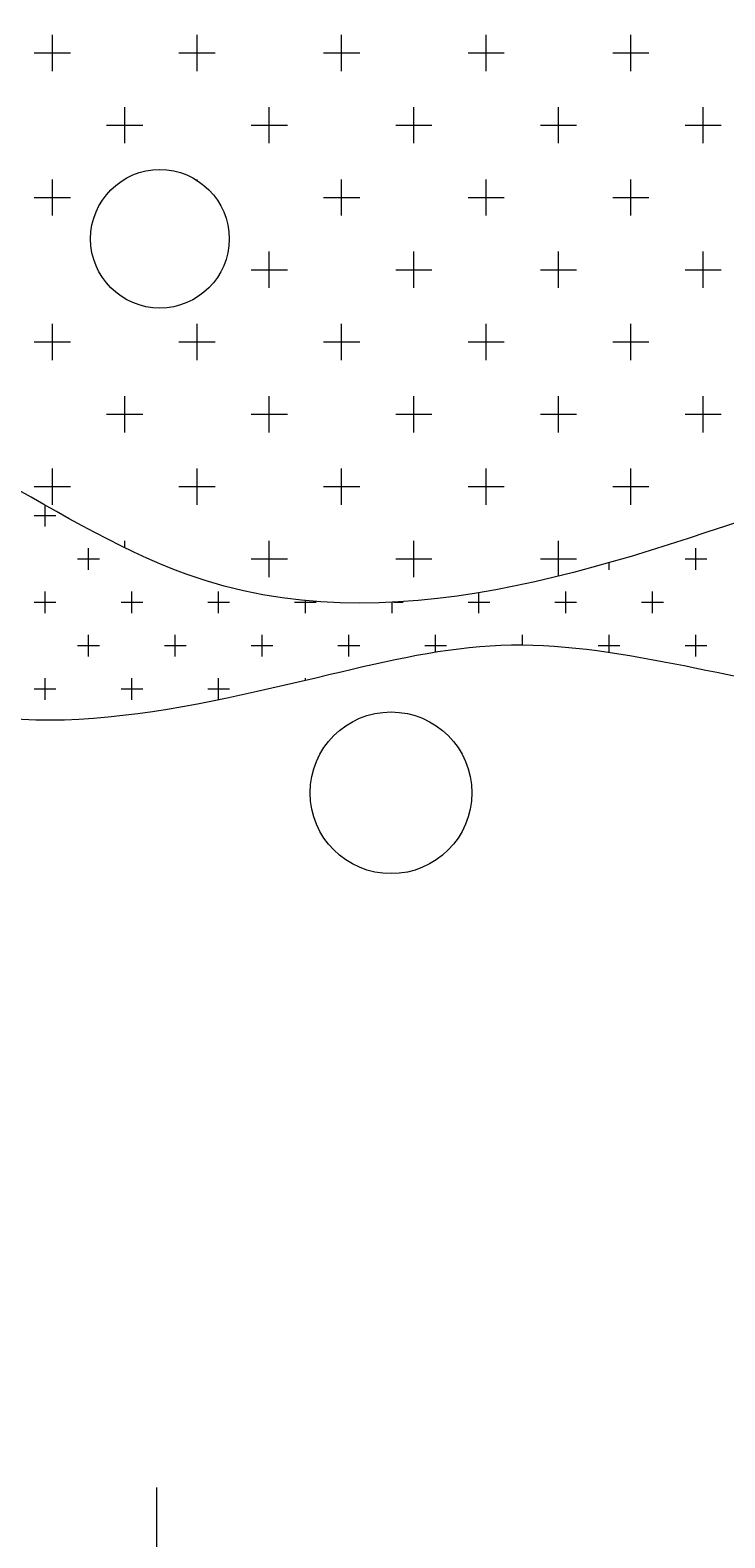
# Model space of a CAD drawing. Units: inches. Extents: x 2330 to 3943, y 1763 to 3461.
# Tile 17 of 40: x 3148 to 3179, y 2593 to 2662. Entities that reach past the tile are written whole.
import ezdxf

# ---------------------------------------------------------------- set-up
doc = ezdxf.new("R2010")
doc.units = ezdxf.units.IN
doc.layers.add('A-ANNO-DIMS', color=2, linetype='Continuous', lineweight=18)
doc.layers.add('A-FURN', color=8, linetype='Continuous', lineweight=13)
doc.styles.get("Standard").update_dxf_attribs({"font": 'arial.ttf'})
doc.dimstyles.get("Standard").update_dxf_attribs({"dimtxt": 0.18, "dimasz": 0.18, "dimexe": 0.18, "dimexo": 0.0625, "dimgap": 0.09, "dimtad": 0, "dimtih": 1, "dimtoh": 1, "dimdec": 4, "dimzin": 0, "dimdsep": 46, "dimtxsty": 'Standard', "dimcen": 0.09, "dimadec": 0, "dimazin": 0, "dimtfac": 1, "dimtdec": 4, "dimtofl": 0, "dimtmove": 0, "dimatfit": 3, "dimfxl": 1, "dimtolj": 1, "dimtzin": 0, "dimarcsym": 0})

# ---------------------------------------------------------------- blocks, each defined once
blk = doc.blocks.new('A$C200C7901')
at = {"linetype": 'ByBlock'}
for p, q in [((0.9504, 1.657), (0.9504, 1.6883)), ((0.9504, 1.657), (0.9504, 1.6883)), ((1.0754, 1.657), (1.0754, 1.6883)), ((1.0754, 1.657), (1.0754, 1.6883)), ((1.2004, 1.657), (1.2004, 1.6883)), ((1.2004, 1.657), (1.2004, 1.6883)), ((1.3254, 1.657), (1.3254, 1.6883)), ((1.3254, 1.657), (1.3254, 1.6883)), ((1.4504, 1.657), (1.4504, 1.6883)), ((1.4504, 1.657), (1.4504, 1.6883)), ((0.9347, 1.6727), (0.966, 1.6727)), ((0.9347, 1.6727), (0.966, 1.6727)), ((1.0597, 1.6727), (1.091, 1.6727)), ((1.0597, 1.6727), (1.091, 1.6727)), ((1.1847, 1.6727), (1.216, 1.6727)), ((1.1847, 1.6727), (1.216, 1.6727)), ((1.3097, 1.6727), (1.341, 1.6727)), ((1.3097, 1.6727), (1.341, 1.6727)), ((1.4347, 1.6727), (1.466, 1.6727)), ((1.4347, 1.6727), (1.466, 1.6727)), ((1.1379, 1.5945), (1.1379, 1.6258)), ((1.1379, 1.5945), (1.1379, 1.6258)), ((1.2629, 1.5945), (1.2629, 1.6258)), ((1.2629, 1.5945), (1.2629, 1.6258)), ((1.3879, 1.5945), (1.3879, 1.6258)), ((1.3879, 1.5945), (1.3879, 1.6258)), ((1.5129, 1.5945), (1.5129, 1.6258)), ((1.5129, 1.5945), (1.5129, 1.6258)), ((0.9972, 1.6102), (1.0285, 1.6102)), ((0.9972, 1.6102), (1.0285, 1.6102)), ((1.1222, 1.6102), (1.1535, 1.6102)), ((1.1222, 1.6102), (1.1535, 1.6102)), ((1.2472, 1.6102), (1.2785, 1.6102)), ((1.2472, 1.6102), (1.2785, 1.6102)), ((1.3722, 1.6102), (1.4035, 1.6102)), ((1.3722, 1.6102), (1.4035, 1.6102)), ((1.4972, 1.6102), (1.5285, 1.6102)), ((1.4972, 1.6102), (1.5285, 1.6102)), ((0.9504, 1.532), (0.9504, 1.5633)), ((0.9504, 1.532), (0.9504, 1.5633)), ((1.2004, 1.532), (1.2004, 1.5633)), ((1.2004, 1.532), (1.2004, 1.5633)), ((1.3254, 1.532), (1.3254, 1.5633)), ((1.3254, 1.532), (1.3254, 1.5633)), ((1.4504, 1.532), (1.4504, 1.5633)), ((1.4504, 1.532), (1.4504, 1.5633)), ((0.9347, 1.5477), (0.966, 1.5477)), ((0.9347, 1.5477), (0.966, 1.5477)), ((1.1847, 1.5477), (1.216, 1.5477)), ((1.1847, 1.5477), (1.216, 1.5477)), ((1.3097, 1.5477), (1.341, 1.5477)), ((1.3097, 1.5477), (1.341, 1.5477)), ((1.4347, 1.5477), (1.466, 1.5477)), ((1.4347, 1.5477), (1.466, 1.5477)), ((1.1379, 1.4695), (1.1379, 1.5008)), ((1.1379, 1.4695), (1.1379, 1.5008)), ((1.2629, 1.4695), (1.2629, 1.5008)), ((1.2629, 1.4695), (1.2629, 1.5008)), ((1.3879, 1.4695), (1.3879, 1.5008)), ((1.3879, 1.4695), (1.3879, 1.5008)), ((1.5129, 1.4695), (1.5129, 1.5008)), ((1.5129, 1.4695), (1.5129, 1.5008)), ((1.1222, 1.4852), (1.1535, 1.4852)), ((1.1222, 1.4852), (1.1535, 1.4852)), ((1.2472, 1.4852), (1.2785, 1.4852)), ((1.2472, 1.4852), (1.2785, 1.4852)), ((1.3722, 1.4852), (1.4035, 1.4852)), ((1.3722, 1.4852), (1.4035, 1.4852)), ((1.4972, 1.4852), (1.5285, 1.4852)), ((1.4972, 1.4852), (1.5285, 1.4852)), ((0.9504, 1.407), (0.9504, 1.4383)), ((0.9504, 1.407), (0.9504, 1.4383)), ((1.0754, 1.407), (1.0754, 1.4383)), ((1.0754, 1.407), (1.0754, 1.4383)), ((1.2004, 1.407), (1.2004, 1.4383)), ((1.2004, 1.407), (1.2004, 1.4383)), ((1.3254, 1.407), (1.3254, 1.4383)), ((1.3254, 1.407), (1.3254, 1.4383)), ((1.4504, 1.407), (1.4504, 1.4383)), ((1.4504, 1.407), (1.4504, 1.4383)), ((0.9347, 1.4227), (0.966, 1.4227)), ((0.9347, 1.4227), (0.966, 1.4227)), ((1.0597, 1.4227), (1.091, 1.4227)), ((1.0597, 1.4227), (1.091, 1.4227)), ((1.1847, 1.4227), (1.216, 1.4227)), ((1.1847, 1.4227), (1.216, 1.4227)), ((1.3097, 1.4227), (1.341, 1.4227)), ((1.3097, 1.4227), (1.341, 1.4227)), ((1.4347, 1.4227), (1.466, 1.4227)), ((1.4347, 1.4227), (1.466, 1.4227)), ((1.0129, 1.3445), (1.0129, 1.3758)), ((1.0129, 1.3445), (1.0129, 1.3758)), ((1.1379, 1.3445), (1.1379, 1.3758)), ((1.1379, 1.3445), (1.1379, 1.3758)), ((1.2629, 1.3445), (1.2629, 1.3758)), ((1.2629, 1.3445), (1.2629, 1.3758)), ((1.3879, 1.3445), (1.3879, 1.3758)), ((1.3879, 1.3445), (1.3879, 1.3758)), ((1.5129, 1.3445), (1.5129, 1.3758)), ((1.5129, 1.3445), (1.5129, 1.3758)), ((0.9972, 1.3602), (1.0285, 1.3602)), ((0.9972, 1.3602), (1.0285, 1.3602)), ((1.1222, 1.3602), (1.1535, 1.3602)), ((1.1222, 1.3602), (1.1535, 1.3602)), ((1.2472, 1.3602), (1.2785, 1.3602)), ((1.2472, 1.3602), (1.2785, 1.3602)), ((1.3722, 1.3602), (1.4035, 1.3602)), ((1.3722, 1.3602), (1.4035, 1.3602)), ((1.4972, 1.3602), (1.5285, 1.3602)), ((1.4972, 1.3602), (1.5285, 1.3602)), ((0.9504, 1.282), (0.9504, 1.3133)), ((0.9504, 1.282), (0.9504, 1.3133)), ((1.0754, 1.282), (1.0754, 1.3133)), ((1.0754, 1.282), (1.0754, 1.3133)), ((1.2004, 1.282), (1.2004, 1.3133)), ((1.2004, 1.282), (1.2004, 1.3133)), ((1.3254, 1.282), (1.3254, 1.3133)), ((1.3254, 1.282), (1.3254, 1.3133)), ((1.4504, 1.282), (1.4504, 1.3133)), ((1.4504, 1.282), (1.4504, 1.3133)), ((0.9347, 1.2977), (0.966, 1.2977)), ((0.9347, 1.2977), (0.966, 1.2977)), ((1.0597, 1.2977), (1.091, 1.2977)), ((1.0597, 1.2977), (1.091, 1.2977)), ((1.1847, 1.2977), (1.216, 1.2977)), ((1.1847, 1.2977), (1.216, 1.2977)), ((1.3097, 1.2977), (1.341, 1.2977)), ((1.3097, 1.2977), (1.341, 1.2977)), ((1.4347, 1.2977), (1.466, 1.2977)), ((1.4347, 1.2977), (1.466, 1.2977)), ((0.9441, 1.2633), (0.9441, 1.2816)), ((0.9441, 1.2633), (0.9441, 1.2816)), ((0.9347, 1.2727), (0.9535, 1.2727)), ((0.9347, 1.2727), (0.9535, 1.2727)), ((0.9816, 1.2258), (0.9816, 1.2445)), ((0.9816, 1.2258), (0.9816, 1.2445)), ((1.0129, 1.2448), (1.0129, 1.2508)), ((1.0129, 1.2448), (1.0129, 1.2508)), ((1.1379, 1.2195), (1.1379, 1.2508)), ((1.1379, 1.2195), (1.1379, 1.2508)), ((1.2629, 1.2195), (1.2629, 1.2508)), ((1.2629, 1.2195), (1.2629, 1.2508)), ((1.3879, 1.2202), (1.3879, 1.2508)), ((1.3879, 1.2202), (1.3879, 1.2508)), ((1.5066, 1.2258), (1.5066, 1.2445)), ((1.5066, 1.2258), (1.5066, 1.2445)), ((0.9722, 1.2352), (0.991, 1.2352)), ((0.9722, 1.2352), (0.991, 1.2352)), ((1.1222, 1.2352), (1.1535, 1.2352)), ((1.1222, 1.2352), (1.1535, 1.2352)), ((1.2472, 1.2352), (1.2785, 1.2352)), ((1.2472, 1.2352), (1.2785, 1.2352)), ((1.3722, 1.2352), (1.4035, 1.2352)), ((1.3722, 1.2352), (1.4035, 1.2352)), ((1.4316, 1.2258), (1.4316, 1.2318)), ((1.4316, 1.2258), (1.4316, 1.2318)), ((1.4972, 1.2352), (1.516, 1.2352)), ((1.4972, 1.2352), (1.516, 1.2352)), ((0.9441, 1.1883), (0.9441, 1.207)), ((0.9441, 1.1883), (0.9441, 1.207)), ((1.0191, 1.1883), (1.0191, 1.207)), ((1.0191, 1.1883), (1.0191, 1.207)), ((1.0941, 1.1883), (1.0941, 1.207)), ((1.0941, 1.1883), (1.0941, 1.207)), ((1.3191, 1.1883), (1.3191, 1.2059)), ((1.3191, 1.1883), (1.3191, 1.2059)), ((1.3941, 1.1883), (1.3941, 1.207)), ((1.3941, 1.1883), (1.3941, 1.207)), ((1.4691, 1.1883), (1.4691, 1.207)), ((1.4691, 1.1883), (1.4691, 1.207)), ((0.9347, 1.1977), (0.9535, 1.1977)), ((0.9347, 1.1977), (0.9535, 1.1977)), ((1.0097, 1.1977), (1.0285, 1.1977)), ((1.0097, 1.1977), (1.0285, 1.1977)), ((1.0847, 1.1977), (1.1035, 1.1977)), ((1.0847, 1.1977), (1.1035, 1.1977)), ((1.1597, 1.1977), (1.1785, 1.1977)), ((1.1597, 1.1977), (1.1785, 1.1977)), ((1.1691, 1.1883), (1.1691, 1.1991)), ((1.1691, 1.1883), (1.1691, 1.1991)), ((1.2441, 1.1883), (1.2441, 1.1976)), ((1.2441, 1.1883), (1.2441, 1.1976)), ((1.2452, 1.1977), (1.2535, 1.1977)), ((1.2452, 1.1977), (1.2535, 1.1977)), ((1.3097, 1.1977), (1.3285, 1.1977)), ((1.3097, 1.1977), (1.3285, 1.1977)), ((1.3847, 1.1977), (1.4035, 1.1977)), ((1.3847, 1.1977), (1.4035, 1.1977)), ((1.4597, 1.1977), (1.4785, 1.1977)), ((1.4597, 1.1977), (1.4785, 1.1977)), ((0.9816, 1.1508), (0.9816, 1.1695)), ((0.9816, 1.1508), (0.9816, 1.1695)), ((1.0566, 1.1508), (1.0566, 1.1695)), ((1.0566, 1.1508), (1.0566, 1.1695)), ((1.1316, 1.1508), (1.1316, 1.1695)), ((1.1316, 1.1508), (1.1316, 1.1695)), ((1.2066, 1.1508), (1.2066, 1.1695)), ((1.2066, 1.1508), (1.2066, 1.1695)), ((1.2816, 1.1547), (1.2816, 1.1695)), ((1.2816, 1.1547), (1.2816, 1.1695)), ((1.3566, 1.1608), (1.3566, 1.1695)), ((1.3566, 1.1608), (1.3566, 1.1695)), ((1.4316, 1.1544), (1.4316, 1.1695)), ((1.4316, 1.1544), (1.4316, 1.1695)), ((1.5066, 1.1508), (1.5066, 1.1695)), ((1.5066, 1.1508), (1.5066, 1.1695)), ((0.9722, 1.1602), (0.991, 1.1602)), ((0.9722, 1.1602), (0.991, 1.1602)), ((1.0472, 1.1602), (1.066, 1.1602)), ((1.0472, 1.1602), (1.066, 1.1602)), ((1.1222, 1.1602), (1.141, 1.1602)), ((1.1222, 1.1602), (1.141, 1.1602)), ((1.1972, 1.1602), (1.216, 1.1602)), ((1.1972, 1.1602), (1.216, 1.1602)), ((1.2722, 1.1602), (1.291, 1.1602)), ((1.2722, 1.1602), (1.291, 1.1602)), ((1.4222, 1.1602), (1.441, 1.1602)), ((1.4222, 1.1602), (1.441, 1.1602)), ((1.4972, 1.1602), (1.516, 1.1602)), ((1.4972, 1.1602), (1.516, 1.1602)), ((0.9347, 1.1227), (0.9535, 1.1227)), ((0.9347, 1.1227), (0.9535, 1.1227)), ((0.9441, 1.1133), (0.9441, 1.132)), ((0.9441, 1.1133), (0.9441, 1.132)), ((1.0097, 1.1227), (1.0285, 1.1227)), ((1.0097, 1.1227), (1.0285, 1.1227)), ((1.0191, 1.1133), (1.0191, 1.132)), ((1.0191, 1.1133), (1.0191, 1.132)), ((1.0847, 1.1227), (1.1035, 1.1227)), ((1.0847, 1.1227), (1.1035, 1.1227)), ((1.0941, 1.1136), (1.0941, 1.132)), ((1.0941, 1.1136), (1.0941, 1.132)), ((1.1691, 1.1303), (1.1691, 1.132)), ((1.1691, 1.1303), (1.1691, 1.132))]:
    blk.add_line(p, q, dxfattribs=at)
for p, q in [((1.0129, 1.5945), (1.0129, 1.6258)), ((1.0129, 1.5945), (1.0129, 1.6258)), ((1.0754, 1.5625), (1.0754, 1.5633)), ((1.0754, 1.5625), (1.0754, 1.5633)), ((1.0407, 0.0275), (1.0407, 0.4323))]:
    blk.add_line(p, q)
for centre, radius in [((1.0433, 1.5119), 0.0599), ((1.2431, 1.0329), 0.0699)]:
    blk.add_circle(centre, radius)
for points, knots in [([(0.4485, 1.7835), (0.4321, 1.7496), (0.4062, 1.6964), (0.49, 1.6713), (0.4719, 1.5969), (0.4123, 1.592), (0.4233, 1.5337), (0.4954, 1.5086), (0.4012, 1.4738), (0.3253, 1.4306), (0.4113, 1.3764), (0.3688, 1.3065), (0.5579, 1.2663), (0.741, 1.4533), (1.1127, 1.1109), (1.4811, 1.2478), (1.7885, 1.3492), (2.0357, 1.1637), (2.0748, 1.2974), (2.0876, 1.349), (2.0192, 1.3805), (2.0564, 1.4298), (2.0588, 1.4846), (1.9759, 1.5349), (2.1004, 1.5845), (2.0397, 1.6519), (1.971, 1.7053), (2.1104, 1.8981), (1.5946, 1.7967), (1.2448, 1.7472), (0.8129, 1.7935), (0.4953, 1.8548), (0.4582, 1.7983), (0.4485, 1.7835)], [0, 0, 0, 0, 88.420092, 139.08588, 204.302936, 239.695496, 287.801042, 327.365471, 412.960499, 463.626286, 552.059846, 584.668336, 662.614915, 940.993281, 1309.926334, 1844.022653, 1996.276242, 2316.43048, 2341.441004, 2404.707416, 2449.463774, 2514.680778, 2538.40571, 2613.031547, 2697.13096, 2760.903931, 2822.692699, 2945.47, 3215.060018, 3725.584917, 4361.974444, 4504.671998, 4555.32777, 4555.32777, 4555.32777, 4555.32777]), ([(0.4856, 1.3429), (0.5504, 1.3182), (0.6715, 1.2721), (0.8374, 1.0498), (1.1164, 1.1183), (1.3878, 1.1816), (1.5888, 1.1102), (1.8403, 1.1127), (1.9415, 1.2178), (2.0032, 1.2819)], [0, 0, 0, 0, 205.411753, 383.654933, 772.067458, 921.644661, 1226.793228, 1388.983508, 1642.292305, 1642.292305, 1642.292305, 1642.292305])]:
    blk.add_open_spline(points, degree=3, knots=knots)
blk.add_open_spline([(0.473, 1.2954), (0.4739, 1.2781), (0.4755, 1.2477), (0.5032, 1.2084), (0.4801, 1.1701), (0.4928, 1.1255), (0.4674, 1.0912), (0.4579, 1.0351), (0.501, 0.9724), (0.4311, 0.8832), (0.4902, 0.8637), (0.4843, 0.8288), (0.4774, 0.7906), (0.4625, 0.7457), (0.459, 0.6999), (0.4816, 0.6664), (0.4748, 0.625), (0.4791, 0.5889), (0.4533, 0.5528), (0.4738, 0.5004), (0.4658, 0.4502), (0.4696, 0.3946), (0.4189, 0.3935), (0.4493, 0.3684), (0.4694, 0.3857), (0.4922, 0.3576), (0.5297, 0.3262), (0.5917, 0.3353), (0.6454, 0.3754), (0.7083, 0.3741), (0.7643, 0.3328), (0.826, 0.346), (0.925, 0.3388), (1.0353, 0.3593), (1.1561, 0.3744), (1.2477, 0.3154), (1.3302, 0.3474), (1.4086, 0.3512), (1.5217, 0.3878), (1.6362, 0.3176), (1.7682, 0.3285), (1.8402, 0.3019), (1.9071, 0.3529), (1.9647, 0.3412), (2.0795, 0.2948), (2.0472, 0.3498), (2.0343, 0.3772), (2.0435, 0.43), (2.0109, 0.5782), (2.0746, 0.4643), (2.0805, 0.584), (2.0084, 0.5979), (2.0343, 0.6846), (2.0344, 0.746), (2.0293, 0.8096), (2.0489, 0.8545), (2.0652, 0.9218), (1.9842, 0.9297), (2.0007, 1.0162), (2.0367, 1.0585), (2.0367, 1.1102), (2.0457, 1.1647), (2.0226, 1.2084), (2.0234, 1.2306), (2.0236, 1.2352)], degree=3, knots=[0, 0, 0, 0, 51.660678, 90.967412, 128.902454, 170.303599, 219.852997, 247.834962, 336.321557, 429.35469, 458.821847, 477.222321, 524.135809, 581.038434, 617.839381, 657.146115, 693.947125, 740.178081, 760.753248, 820.731705, 885.133458, 928.777044, 953.563729, 976.574207, 995.553042, 1018.563482, 1064.584401, 1147.951297, 1174.787598, 1266.851571, 1308.018447, 1377.066427, 1441.511314, 1608.245014, 1714.11869, 1792.771707, 1913.247991, 1954.931389, 2029.864445, 2259.189419, 2305.221512, 2429.507982, 2456.344283, 2543.92595, 2627.925037, 2662.96218, 2687.736879, 2719.937755, 2839.540991, 2875.47895, 2953.681041, 2993.270313, 3066.872333, 3154.395764, 3200.397042, 3248.426375, 3312.828127, 3347.881398, 3444.484026, 3481.577522, 3518.665244, 3592.267265, 3644.719162, 3658.519501, 3658.519501, 3658.519501, 3658.519501], dxfattribs=at)
blk = doc.blocks.new('*D95')
at = {"layer": 'A-ANNO-DIMS', "color": 0, "lineweight": -2, "transparency": 16777216}
for p, q in [((3105.603, 2727.687), (3105.783, 2727.687)), ((3105.693, 2727.597), (3105.693, 2727.777)), ((3606.312, 2659.69), (3418.758, 2685.165))]:
    blk.add_line(p, q, dxfattribs=at)
at = {"layer": 'A-ANNO-DIMS', "color": 0, "transparency": 16777216}
blk.add_solid([(3418.762, 2685.195), (3418.754, 2685.135), (3418.58, 2685.189)], dxfattribs=at)
at = {"layer": 'Defpoints', "color": 0, "transparency": 16777216}
for p in [(3105.693, 2727.687), (3418.58, 2685.189)]:
    blk.add_point(p, dxfattribs=at)
at = {"layer": 'A-ANNO-DIMS', "color": 0, "transparency": 16777216, "insert": (3606.862, 2659.69), "char_height": 0.18, "attachment_point": 5}
blk.add_mtext('\\A1;R315.76', dxfattribs=at)
blk = doc.blocks.new('*D97')
at = {"layer": 'A-ANNO-DIMS', "color": 0, "lineweight": -2, "transparency": 16777216}
for p, q in [((3105.603, 2727.687), (3105.783, 2727.687)), ((3105.693, 2727.597), (3105.693, 2727.777)), ((3589.166, 2615.071), (3408.039, 2657.261))]:
    blk.add_line(p, q, dxfattribs=at)
at = {"layer": 'A-ANNO-DIMS', "color": 0, "transparency": 16777216}
blk.add_solid([(3408.046, 2657.29), (3408.032, 2657.232), (3407.864, 2657.302)], dxfattribs=at)
at = {"layer": 'Defpoints', "color": 0, "transparency": 16777216}
for p in [(3105.693, 2727.687), (3407.864, 2657.302)]:
    blk.add_point(p, dxfattribs=at)
at = {"layer": 'A-ANNO-DIMS', "color": 0, "transparency": 16777216, "insert": (3589.911, 2615.071), "char_height": 0.18, "attachment_point": 5}
blk.add_mtext('\\A1;2X R310.26', dxfattribs=at)
blk = doc.blocks.new('*D98')
at = {"layer": 'A-ANNO-DIMS', "color": 0, "lineweight": -2, "transparency": 16777216}
for p, q in [((3105.603, 2727.687), (3105.783, 2727.687)), ((3105.693, 2727.597), (3105.693, 2727.777)), ((3519.334, 2463.489), (3364.371, 2562.466)), ((3519.514, 2463.489), (3519.334, 2463.489))]:
    blk.add_line(p, q, dxfattribs=at)
at = {"layer": 'A-ANNO-DIMS', "color": 0, "transparency": 16777216}
blk.add_solid([(3364.387, 2562.491), (3364.355, 2562.441), (3364.219, 2562.563)], dxfattribs=at)
at = {"layer": 'Defpoints', "color": 0, "transparency": 16777216}
for p in [(3105.693, 2727.687), (3364.219, 2562.563)]:
    blk.add_point(p, dxfattribs=at)
at = {"layer": 'A-ANNO-DIMS', "color": 0, "transparency": 16777216, "insert": (3520.257, 2463.489), "char_height": 0.18, "attachment_point": 5}
blk.add_mtext('\\A1;3X R306.76', dxfattribs=at)

msp = doc.modelspace()

# ---------------------------------------------------------------- block references
at = {"layer": 'A-FURN', "xscale": 52.5181391560459, "yscale": 52.5181391560459, "zscale": 52.5181391560459}
msp.add_blockref('A$C200C7901', (3098.8053, 2572.8601), dxfattribs=at)

# ---------------------------------------------------------------- dimensions: what is measured, and where the dimension line sits
at = {"layer": 'A-ANNO-DIMS'}
dim = msp.add_radius_dim(center=(3105.6935, 2727.6869), mpoint=(3418.58, 2685.189), dimstyle='Standard', override={"dimdec": 2, "dimlfac": 1, "dimrnd": 0, "dimzin": 0, "dimdsep": 46, "dimlunit": 2}, dxfattribs=at)
dim.commit()
dim.dimension.update_dxf_attribs({"geometry": '*D95', "text_midpoint": (3606.3119, 2659.6902), "dimtype": 164})
for mpoint, text, picture, middle in [((3407.8638, 2657.302), '2X <>', '*D97', (3589.166, 2615.0711)), ((3364.219, 2562.563), '3X <>', '*D98', (3520.2574, 2463.4886))]:
    dim = msp.add_radius_dim(center=(3105.6935, 2727.6869), mpoint=mpoint, text=text, dimstyle='Standard', override={"dimdec": 2, "dimlfac": 1, "dimrnd": 0, "dimzin": 0, "dimdsep": 46, "dimlunit": 2}, dxfattribs=at)
    dim.commit()
    dim.dimension.update_dxf_attribs({"geometry": picture, "text_midpoint": middle, "dimtype": 164})

doc.saveas('drawing.dxf')
